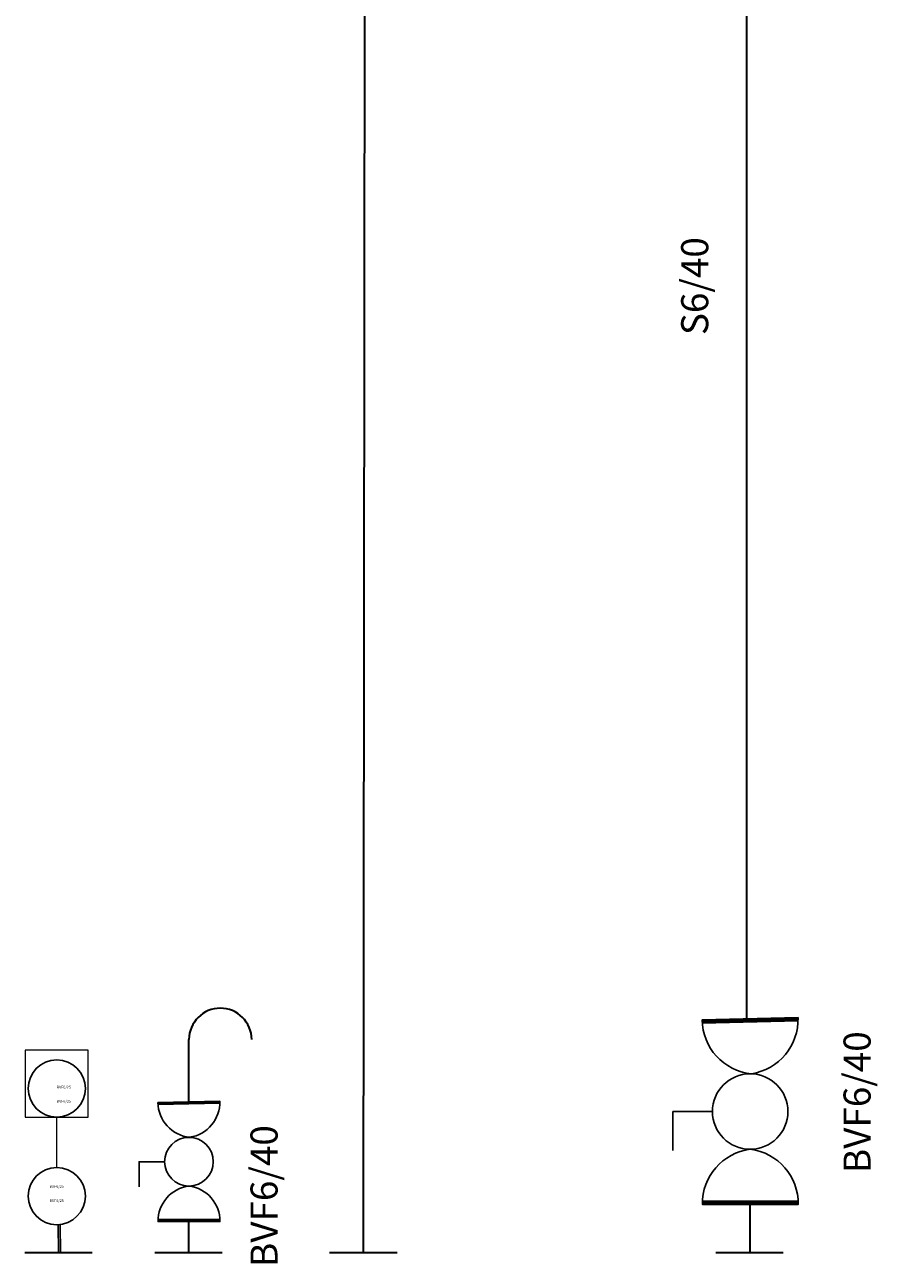
# Model space of a CAD drawing. Units: millimetres. Extents: x 353872 to 441597, y 126154 to 187356.
# Tile 14 of 28: x 395421 to 398510, y 149282 to 153772. Entities that reach past the tile are written whole.
import ezdxf

# ---------------------------------------------------------------- set-up
doc = ezdxf.new("R2010")
doc.units = ezdxf.units.MM
for name, color, linetype, lineweight in [('P-ANNO-SYMB', 7, 'Continuous', 18), ('P-ANNO-TEXT', 7, 'Continuous', 25), ('P-INST', 6, 'Continuous', 25), ('P-PIPE', 3, 'Continuous', 35), ('P-VALV', 2, 'Continuous', 25)]:
    doc.layers.add(name, color=color, linetype=linetype, lineweight=lineweight)
doc.styles.get("Standard").update_dxf_attribs({"font": 'arial.ttf'})

# ---------------------------------------------------------------- blocks, each defined once
blk = doc.blocks.new('VALVE-B')
for points in [[(0, 4), (0, 0), (347.3, 0), (347.3, 5.4)], [(0, 3.9), (0, 3.9), (343.4, 3.9), (347.3, 3.9)], [(0.1, 7.9), (347.2, 7.9)], [(0.2, 12), (347.1, 12.1)]]:
    blk.add_lwpolyline(points)
for centre, radius, start, end in [((199.1, 2), 199.2, 97.3612, 180.5798), ((148.9, 2.7), 198.4, 359.2193, 82.8397)]:
    blk.add_arc(centre, radius, start, end)
blk = doc.blocks.new('VALVE-C')
for points in [[(0, 2.6), (0, 0), (224, 0), (224, 3.5)], [(0, 2.5), (0, 2.5), (221.5, 2.5), (224, 2.5)], [(0.1, 5.1), (224, 5.1)], [(0.2, 7.8), (223.9, 7.8)]]:
    blk.add_lwpolyline(points)
for centre, radius, start, end in [((128.5, 1.3), 128.5, 97.3612, 180.5798), ((96.1, 1.7), 128, 359.2193, 82.8397)]:
    blk.add_arc(centre, radius, start, end)

msp = doc.modelspace()

# ---------------------------------------------------------------- linework, layer by layer
at = {"layer": 'P-ANNO-SYMB'}
msp.add_line((395537.23, 149629.25), (395537.23, 149811.88), dxfattribs=at)
msp.add_lwpolyline([(395651.56, 150054.49), (395422.91, 150054.49), (395422.91, 149811.88), (395651.56, 149811.88)], close=True, dxfattribs=at)
at = {"layer": 'P-INST'}
for p, q in [((395542.05, 149423.15), (395543.84, 149319.73)), ((395549.11, 149423.28), (395550.91, 149319.85))]:
    msp.add_line(p, q, dxfattribs=at)
for centre in [(395537.23, 149915.56), (395537.23, 149525.57)]:
    msp.add_circle(centre, 103.68, dxfattribs=at)
at = {"layer": 'P-PIPE'}
for p, q in [((396659.16, 160948.84), (396648.15, 149319.73)), ((398036.88, 156699.54), (398036.88, 150168.41)), ((396016.48, 149867.25), (396016.48, 150093.02)), ((398048.48, 149495.52), (398048.48, 149319.73)), ((396015.22, 149433.14), (396015.22, 149319.73)), ((395666.22, 149319.73), (395421.46, 149319.73)), ((396136.94, 149319.73), (395892.18, 149319.73)), ((396770.53, 149319.73), (396525.77, 149319.73)), ((398169.84, 149319.73), (397925.08, 149319.73))]:
    msp.add_line(p, q, dxfattribs=at)
msp.add_arc((396130.07, 150093.02), 113.59, 0, 180, dxfattribs=at)
at = {"layer": 'P-VALV'}
for points in [[(397913.12, 149831.97), (397769.82, 149831.97), (397769.82, 149691.27)], [(395927.89, 149650.19), (395835.44, 149650.19), (395835.44, 149559.43)]]:
    msp.add_lwpolyline(points, dxfattribs=at)
for centre, radius in [((398049.97, 149831.97), 136.85), ((396016.18, 149650.19), 88.29)]:
    msp.add_circle(centre, radius, dxfattribs=at)

# ---------------------------------------------------------------- block references
for name, p, rotation in [('VALVE-B', (398223.3, 150172.35), 181.3019170021883), ('VALVE-C', (396128, 149869.79), 181.3019170023652)]:
    msp.add_blockref(name, p, dxfattribs=dict(at, rotation=rotation))
for name, p in [('VALVE-B', (397876.8, 149495.52)), ('VALVE-C', (395904.46, 149433.14))]:
    msp.add_blockref(name, p, dxfattribs=at)

# ---------------------------------------------------------------- texts
at = {"layer": 'P-ANNO-TEXT'}
for s, p in [('S6/40', (397898.04, 152646.61)), ('BVF6/40', (398486.4, 149608.96)), ('BVF6/40', (396337.48, 149268.59))]:
    msp.add_text(s, height=98.09, rotation=90, dxfattribs=at).set_placement(p)
for p in [(395537.23, 149915.56), (395537.23, 149864.44), (395511.21, 149555.16), (395511.21, 149504.04)]:
    msp.add_text('BVF6/25', height=9.835, dxfattribs=at).set_placement(p)

doc.saveas('drawing.dxf')
